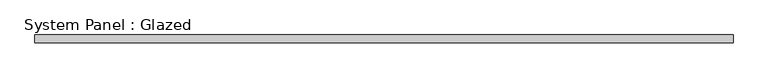
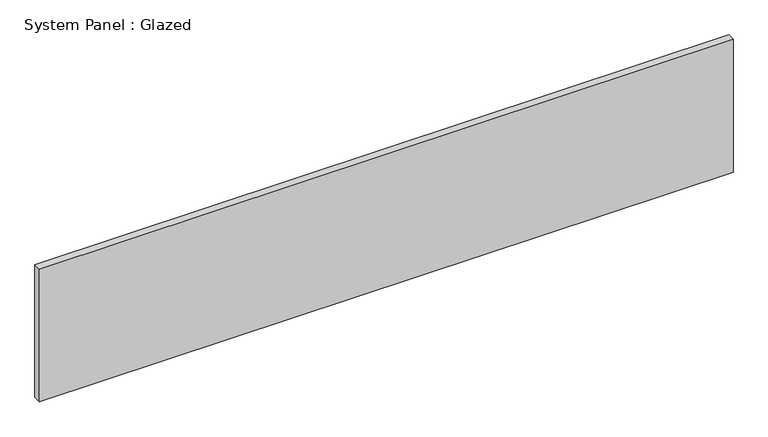
"""IFC4 building model written with IfcOpenShell, lengths in millimetres: plate geometry, System Panel : Glazed."""

from ifc_helpers import new_model, si_unit, origin, origin_with_axes, place, context, project, spatial, polyline, outline, extrude, source, transform, mapped, element, save


def system_panel_glazed_f70c9889(model_context):
    return source(origin(), model_context, "Body", "SweptSolid", [
        extrude(outline(polyline([(1120.775, 19.05), (-1120.775, 19.05), (-1120.775, 44.45), (1120.775, 44.45), (1120.775, 19.05)])), origin_with_axes(), (0.0, 0.0, 1.0), 453.786674),
    ])


if __name__ == "__main__":
    model = new_model("IFC4")
    model_context = context("Model", 3, world=origin())
    ifc_project = project(units=[si_unit("LENGTHUNIT", "METRE", prefix="MILLI")], contexts=[model_context])
    site = spatial("IfcSite", under=ifc_project)
    building = spatial("IfcBuilding", under=site)
    placement = place(None, origin())
    system_panel_glazed_shape = system_panel_glazed_f70c9889(model_context)
    element("IfcPlate", 1, ObjectType="System Panel : Glazed", at=placement, inside=building, context=model_context, shape_type="MappedRepresentation", body=[
        mapped(system_panel_glazed_shape, transform((0.0, 0.0, 0.0), x_axis=(1.0, 0.0, 0.0), y_axis=(0.0, 1.0, 0.0), z_axis=(0.0, 0.0, 1.0))),
    ])
    save(model, "model.ifc")

# Revit data of these elements
# Type "System Panel : Glazed"
#   Construction Type Id = "GSP4R"
#   Analytic Construction = "1/8 in Pilkington single glazing"
#   Visual Light Transmittance = 0.9
#   Solar Heat Gain Coefficient = 0.86
#   Heat Transfer Coefficient (U) = 1.18115 BTU/(h·ft²·°F)
#   Define Thermal Properties by = 1
# Element 1 (IfcPlate, "System Panel : Glazed")
#   Materials on its faces: "Glass"
# Materials
#   "Glass": class "Glass", colour RGB 0 128 192, transparency 0.75, Description = "Soda Lime Glass", Cost = 0
